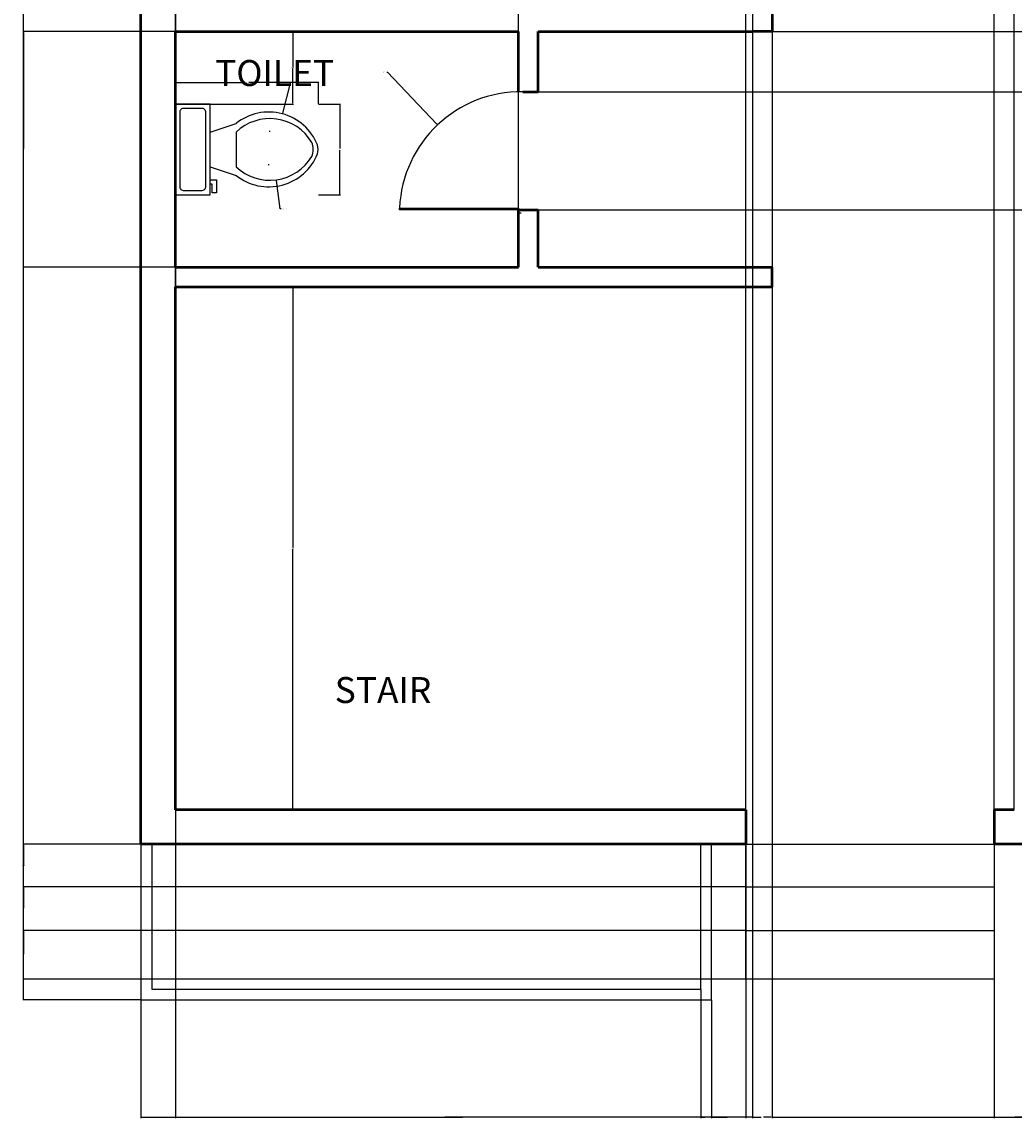
# Model space of a CAD drawing. Units: inches. Extents: x 2907 to 3328, y 1715 to 2286.
# Tile 1 of 5: x 2907 to 3137, y 1715 to 1969. Entities that reach past the tile are written whole.
import ezdxf

# ---------------------------------------------------------------- set-up
doc = ezdxf.new("R2010")
doc.units = ezdxf.units.IN
for name, color, linetype, lineweight in [('A-ANNO-DIMS', 2, 'Continuous', 18), ('A-AREA-IDEN', 7, 'Continuous', 25), ('A-DOOR', 3, 'Continuous', 25), ('A-FLOR-FIXT', 9, 'Continuous', 25), ('A-FLOR-OTLN', 7, 'Continuous', 25), ('A-FLOR-STRS', 7, 'Continuous', 25), ('A-WALL', 7, 'Continuous', 50)]:
    doc.layers.add(name, color=color, linetype=linetype, lineweight=lineweight)
doc.styles.get("Standard").update_dxf_attribs({"font": 'arial.ttf'})
doc.dimstyles.get("Standard").update_dxf_attribs({"dimtxt": 0.18, "dimasz": 0.18, "dimexe": 0.18, "dimexo": 0.0625, "dimgap": 0.09, "dimtad": 0, "dimtih": 1, "dimtoh": 1, "dimdec": 4, "dimzin": 0, "dimdsep": 46, "dimtxsty": 'Standard', "dimcen": 0.09, "dimadec": 0, "dimazin": 0, "dimtfac": 1, "dimtdec": 4, "dimtofl": 0, "dimtmove": 0, "dimatfit": 3, "dimfxl": 1, "dimtolj": 1, "dimtzin": 0, "dimarcsym": 0})

# ---------------------------------------------------------------- blocks, each defined once
blk = doc.blocks.new('Toilet - top')
for p, q in [((9.5, -6), (9.5, -2)), ((-10, -8.5), (-8, -8.5)), ((-10, -9.5), (-10, -8.5)), ((-7, -9.5), (-10, -9.5)), ((-8, -8.5), (-8, -8)), ((-7, -8), (-7, -9.5)), ((-4, -8), (-6, -14)), ((4, -8), (6, -14)), ((4, -14), (-4, -14))]:
    blk.add_line(p, q)
blk.add_lwpolyline([(10.5, -8), (10.5, 0), (-10.5, 0), (-10.5, -8)], close=True)
for points in [[(-9.5, -2), (-9.5, -6)], [(8.5, -1), (-8.5, -1)], [(-8.5, -7), (8.5, -7)]]:
    blk.add_lwpolyline(points)
for centre, radius, start, end in [((-8.62, -1.88), 0.884, 81.8699, 188.1301), ((8.62, -1.88), 0.884, 351.8699, 98.1301), ((-8.62, -6.12), 0.884, 171.8699, 278.1301), ((8.62, -6.12), 0.884, 261.8699, 8.1301), ((3.52, -21.58), 12.17, 141.4691, 247.9714), ((4.2, -21.82), 11.33, 136.3677, 238.9468), ((-3.52, -21.58), 12.17, 292.0284, 38.5307), ((-4.2, -21.82), 11.33, 301.053, 43.6321), ((0, -27.88), 4, 245.7318, 294.2682), ((0, -29), 4, 254.8605, 285.1395)]:
    blk.add_arc(centre, radius, start, end)
blk = doc.blocks.new('*D11')
at = {"layer": 'A-ANNO-DIMS', "color": 0, "lineweight": -2, "transparency": 16777216}
for p, q in [((2942.59, 1950.14), (2942.59, 1955.22)), ((2975.64, 1950.14), (2975.64, 1955.22)), ((2942.77, 1955.04), (2958.65, 1955.04)), ((2975.46, 1955.04), (2959.58, 1955.04))]:
    blk.add_line(p, q, dxfattribs=at)
at = {"layer": 'A-ANNO-DIMS', "color": 0, "transparency": 16777216}
for points in [[(2942.77, 1955.07), (2942.77, 1955.01), (2942.59, 1955.04)], [(2975.46, 1955.07), (2975.46, 1955.01), (2975.64, 1955.04)]]:
    blk.add_solid(points, dxfattribs=at)
at = {"layer": 'Defpoints', "color": 0, "transparency": 16777216}
for p in [(2942.59, 1955.04), (2942.59, 1950.08), (2975.64, 1950.08)]:
    blk.add_point(p, dxfattribs=at)
at = {"layer": 'A-ANNO-DIMS', "color": 0, "transparency": 16777216, "insert": (2959.11, 1955.04), "char_height": 0.18, "attachment_point": 5}
blk.add_mtext('\\A1;WC 33', dxfattribs=at)
blk = doc.blocks.new('*D12')
at = {"layer": 'A-ANNO-DIMS', "color": 0, "lineweight": -2, "transparency": 16777216}
for p, q in [((2975.7, 1950.08), (2980.77, 1950.08)), ((2980.59, 1949.9), (2980.59, 1939.76)), ((2980.59, 1929.26), (2980.59, 1939.4)), ((2975.7, 1929.08), (2980.77, 1929.08))]:
    blk.add_line(p, q, dxfattribs=at)
at = {"layer": 'A-ANNO-DIMS', "color": 0, "transparency": 16777216}
for points in [[(2980.56, 1949.9), (2980.62, 1949.9), (2980.59, 1950.08)], [(2980.56, 1929.26), (2980.62, 1929.26), (2980.59, 1929.08)]]:
    blk.add_solid(points, dxfattribs=at)
at = {"layer": 'Defpoints', "color": 0, "transparency": 16777216}
for p in [(2975.64, 1950.08), (2980.59, 1950.08), (2975.64, 1929.08)]:
    blk.add_point(p, dxfattribs=at)
at = {"layer": 'A-ANNO-DIMS', "color": 0, "transparency": 16777216, "insert": (2980.59, 1939.58), "char_height": 0.18, "attachment_point": 5}
blk.add_mtext('\\A1;21', dxfattribs=at)
blk = doc.blocks.new('*D14')
at = {"layer": 'A-ANNO-DIMS', "color": 0, "lineweight": -2, "transparency": 16777216}
for p, q in [((2934.53, 2258.83), (2907.26, 2258.83)), ((2907.44, 2258.65), (2907.44, 2001.01)), ((2907.44, 1743.01), (2907.44, 2000.65)), ((2934.53, 1742.83), (2907.26, 1742.83))]:
    blk.add_line(p, q, dxfattribs=at)
at = {"layer": 'A-ANNO-DIMS', "color": 0, "transparency": 16777216}
for points in [[(2907.41, 2258.65), (2907.47, 2258.65), (2907.44, 2258.83)], [(2907.41, 1743.01), (2907.47, 1743.01), (2907.44, 1742.83)]]:
    blk.add_solid(points, dxfattribs=at)
at = {"layer": 'Defpoints', "color": 0, "transparency": 16777216}
for p in [(2907.44, 2258.83), (2934.59, 2258.83), (2934.59, 1742.83)]:
    blk.add_point(p, dxfattribs=at)
at = {"layer": 'A-ANNO-DIMS', "color": 0, "transparency": 16777216, "insert": (2907.44, 2000.83), "char_height": 0.18, "attachment_point": 5}
blk.add_mtext('\\A1;516', dxfattribs=at)
blk = doc.blocks.new('*D16')
at = {"layer": 'A-ANNO-DIMS', "color": 0, "lineweight": -2, "transparency": 16777216}
for p, q in [((2942.59, 2250.77), (2942.59, 1715.5)), ((3076.09, 2250.77), (3076.09, 1715.5)), ((2942.77, 1715.68), (3008.95, 1715.68)), ((3075.91, 1715.68), (3009.73, 1715.68))]:
    blk.add_line(p, q, dxfattribs=at)
at = {"layer": 'A-ANNO-DIMS', "color": 0, "transparency": 16777216}
for points in [[(2942.77, 1715.71), (2942.77, 1715.65), (2942.59, 1715.68)], [(3075.91, 1715.71), (3075.91, 1715.65), (3076.09, 1715.68)]]:
    blk.add_solid(points, dxfattribs=at)
at = {"layer": 'Defpoints', "color": 0, "transparency": 16777216}
for p in [(2942.59, 2250.83), (3076.09, 2250.83), (3076.09, 1715.68)]:
    blk.add_point(p, dxfattribs=at)
at = {"layer": 'A-ANNO-DIMS', "color": 0, "transparency": 16777216, "insert": (3009.34, 1715.68), "char_height": 0.18, "attachment_point": 5}
blk.add_mtext('\\A1;133.5', dxfattribs=at)
blk = doc.blocks.new('*D17')
at = {"layer": 'A-ANNO-DIMS', "color": 0, "lineweight": -2, "transparency": 16777216}
for p, q in [((3080.59, 2250.77), (3080.59, 1715.5)), ((3192.09, 2250.77), (3192.09, 1715.5)), ((3080.77, 1715.68), (3135.95, 1715.68)), ((3191.91, 1715.68), (3136.73, 1715.68))]:
    blk.add_line(p, q, dxfattribs=at)
at = {"layer": 'A-ANNO-DIMS', "color": 0, "transparency": 16777216}
for points in [[(3080.77, 1715.71), (3080.77, 1715.65), (3080.59, 1715.68)], [(3191.91, 1715.71), (3191.91, 1715.65), (3192.09, 1715.68)]]:
    blk.add_solid(points, dxfattribs=at)
at = {"layer": 'Defpoints', "color": 0, "transparency": 16777216}
for p in [(3080.59, 2250.83), (3192.09, 2250.83), (3192.09, 1715.68)]:
    blk.add_point(p, dxfattribs=at)
at = {"layer": 'A-ANNO-DIMS', "color": 0, "transparency": 16777216, "insert": (3136.34, 1715.68), "char_height": 0.18, "attachment_point": 5}
blk.add_mtext('\\A1;111.5', dxfattribs=at)
blk = doc.blocks.new('*D27')
at = {"layer": 'A-ANNO-DIMS', "color": 0, "lineweight": -2, "transparency": 16777216}
for p, q in [((2942.53, 1966.83), (2907.26, 1966.83)), ((2907.44, 1966.65), (2907.44, 1939.76)), ((2907.44, 1912.51), (2907.44, 1939.4)), ((2942.53, 1912.33), (2907.26, 1912.33))]:
    blk.add_line(p, q, dxfattribs=at)
at = {"layer": 'A-ANNO-DIMS', "color": 0, "transparency": 16777216}
for points in [[(2907.41, 1966.65), (2907.47, 1966.65), (2907.44, 1966.83)], [(2907.41, 1912.51), (2907.47, 1912.51), (2907.44, 1912.33)]]:
    blk.add_solid(points, dxfattribs=at)
at = {"layer": 'Defpoints', "color": 0, "transparency": 16777216}
for p in [(2907.44, 1966.83), (2942.59, 1966.83), (2942.59, 1912.33)]:
    blk.add_point(p, dxfattribs=at)
at = {"layer": 'A-ANNO-DIMS', "color": 0, "transparency": 16777216, "insert": (2907.44, 1939.58), "char_height": 0.18, "attachment_point": 5}
blk.add_mtext('\\A1;54.5', dxfattribs=at)
blk = doc.blocks.new('*D31')
at = {"layer": 'A-ANNO-DIMS', "color": 0, "lineweight": -2, "transparency": 16777216}
for p, q in [((2942.59, 1912.39), (2942.59, 2286.16)), ((2942.77, 2285.98), (2981.88, 2285.98)), ((3021.78, 2285.98), (2982.67, 2285.98)), ((3021.96, 1912.39), (3021.96, 2286.16))]:
    blk.add_line(p, q, dxfattribs=at)
at = {"layer": 'A-ANNO-DIMS', "color": 0, "transparency": 16777216}
for points in [[(2942.77, 2286.01), (2942.77, 2285.95), (2942.59, 2285.98)], [(3021.78, 2286.01), (3021.78, 2285.95), (3021.96, 2285.98)]]:
    blk.add_solid(points, dxfattribs=at)
at = {"layer": 'Defpoints', "color": 0, "transparency": 16777216}
for p in [(3021.96, 2285.98), (2942.59, 1912.33), (3021.96, 1912.33)]:
    blk.add_point(p, dxfattribs=at)
at = {"layer": 'A-ANNO-DIMS', "color": 0, "transparency": 16777216, "insert": (2982.27, 2285.98), "char_height": 0.18, "attachment_point": 5}
blk.add_mtext('\\A1;79.37', dxfattribs=at)
blk = doc.blocks.new('*D33')
at = {"layer": 'A-ANNO-DIMS', "color": 0, "lineweight": -2, "transparency": 16777216}
for p, q in [((2934.59, 1778.77), (2934.59, 1715.5)), ((3074.5, 1778.77), (3074.5, 1715.5)), ((2934.77, 1715.68), (3004.16, 1715.68)), ((3074.32, 1715.68), (3004.93, 1715.68))]:
    blk.add_line(p, q, dxfattribs=at)
at = {"layer": 'A-ANNO-DIMS', "color": 0, "transparency": 16777216}
for points in [[(2934.77, 1715.71), (2934.77, 1715.65), (2934.59, 1715.68)], [(3074.32, 1715.71), (3074.32, 1715.65), (3074.5, 1715.68)]]:
    blk.add_solid(points, dxfattribs=at)
at = {"layer": 'Defpoints', "color": 0, "transparency": 16777216}
for p in [(2934.59, 1778.83), (3074.5, 1778.83), (3074.5, 1715.68)]:
    blk.add_point(p, dxfattribs=at)
at = {"layer": 'A-ANNO-DIMS', "color": 0, "transparency": 16777216, "insert": (3004.54, 1715.68), "char_height": 0.18, "attachment_point": 5}
blk.add_mtext('\\A1;139.9', dxfattribs=at)
blk = doc.blocks.new('*D34')
at = {"layer": 'A-ANNO-DIMS', "color": 0, "lineweight": -2, "transparency": 16777216}
for p, q in [((3074.5, 1778.89), (3074.5, 2286.16)), ((3074.68, 2285.98), (3102.84, 2285.98)), ((3131.79, 2285.98), (3103.63, 2285.98)), ((3131.97, 1778.89), (3131.97, 2286.16))]:
    blk.add_line(p, q, dxfattribs=at)
at = {"layer": 'A-ANNO-DIMS', "color": 0, "transparency": 16777216}
for points in [[(3074.68, 2286.01), (3074.68, 2285.95), (3074.5, 2285.98)], [(3131.79, 2286.01), (3131.79, 2285.95), (3131.97, 2285.98)]]:
    blk.add_solid(points, dxfattribs=at)
at = {"layer": 'Defpoints', "color": 0, "transparency": 16777216}
for p in [(3131.97, 2285.98), (3074.5, 1778.83), (3131.97, 1778.83)]:
    blk.add_point(p, dxfattribs=at)
at = {"layer": 'A-ANNO-DIMS', "color": 0, "transparency": 16777216, "insert": (3103.24, 2285.98), "char_height": 0.18, "attachment_point": 5}
blk.add_mtext('\\A1;57.47', dxfattribs=at)
blk = doc.blocks.new('*D35')
at = {"layer": 'A-ANNO-DIMS', "color": 0, "lineweight": -2, "transparency": 16777216}
for p, q in [((3131.97, 1778.77), (3131.97, 1715.5)), ((3196.08, 1778.77), (3196.08, 1715.5)), ((3132.15, 1715.68), (3163.72, 1715.68)), ((3195.9, 1715.68), (3164.33, 1715.68))]:
    blk.add_line(p, q, dxfattribs=at)
at = {"layer": 'A-ANNO-DIMS', "color": 0, "transparency": 16777216}
for points in [[(3132.15, 1715.71), (3132.15, 1715.65), (3131.97, 1715.68)], [(3195.9, 1715.71), (3195.9, 1715.65), (3196.08, 1715.68)]]:
    blk.add_solid(points, dxfattribs=at)
at = {"layer": 'Defpoints', "color": 0, "transparency": 16777216}
for p in [(3131.97, 1778.83), (3196.08, 1778.83), (3196.08, 1715.68)]:
    blk.add_point(p, dxfattribs=at)
at = {"layer": 'A-ANNO-DIMS', "color": 0, "transparency": 16777216, "insert": (3164.03, 1715.68), "char_height": 0.18, "attachment_point": 5}
blk.add_mtext('\\A1;64.1', dxfattribs=at)
blk = doc.blocks.new('*D40')
at = {"layer": 'A-ANNO-DIMS', "color": 0, "lineweight": -2, "transparency": 16777216}
for p, q in [((3026.52, 1952.9), (3327.92, 1952.9)), ((3327.74, 1952.72), (3327.74, 1939.45)), ((3327.74, 1925.82), (3327.74, 1939.09)), ((3026.52, 1925.64), (3327.92, 1925.64))]:
    blk.add_line(p, q, dxfattribs=at)
at = {"layer": 'A-ANNO-DIMS', "color": 0, "transparency": 16777216}
for points in [[(3327.71, 1952.72), (3327.77, 1952.72), (3327.74, 1952.9)], [(3327.71, 1925.82), (3327.77, 1925.82), (3327.74, 1925.64)]]:
    blk.add_solid(points, dxfattribs=at)
at = {"layer": 'Defpoints', "color": 0, "transparency": 16777216}
for p in [(3026.46, 1952.9), (3327.74, 1952.9), (3026.46, 1925.64)]:
    blk.add_point(p, dxfattribs=at)
at = {"layer": 'A-ANNO-DIMS', "color": 0, "transparency": 16777216, "insert": (3327.74, 1939.27), "char_height": 0.18, "attachment_point": 5}
blk.add_mtext('\\A1;27.27', dxfattribs=at)
blk = doc.blocks.new('*D41')
at = {"layer": 'A-ANNO-DIMS', "color": 0, "lineweight": -2, "transparency": 16777216}
for p, q in [((3026.52, 1966.83), (3327.92, 1966.83)), ((3327.74, 1966.65), (3327.74, 1960.05)), ((3327.74, 1953.08), (3327.74, 1959.68)), ((3026.52, 1952.9), (3327.92, 1952.9))]:
    blk.add_line(p, q, dxfattribs=at)
at = {"layer": 'A-ANNO-DIMS', "color": 0, "transparency": 16777216}
for points in [[(3327.71, 1966.65), (3327.77, 1966.65), (3327.74, 1966.83)], [(3327.71, 1953.08), (3327.77, 1953.08), (3327.74, 1952.9)]]:
    blk.add_solid(points, dxfattribs=at)
at = {"layer": 'Defpoints', "color": 0, "transparency": 16777216}
for p in [(3026.46, 1966.83), (3327.74, 1966.83), (3026.46, 1952.9)]:
    blk.add_point(p, dxfattribs=at)
at = {"layer": 'A-ANNO-DIMS', "color": 0, "transparency": 16777216, "insert": (3327.74, 1959.87), "char_height": 0.18, "attachment_point": 5}
blk.add_mtext('\\A1;13.927', dxfattribs=at)
blk = doc.blocks.new('*D47')
at = {"layer": 'A-ANNO-DIMS', "color": 0, "lineweight": -2, "transparency": 16777216}
for p, q in [((3076.09, 2250.77), (3076.09, 1715.5)), ((3080.59, 2250.77), (3080.59, 1715.5)), ((3076.27, 1715.68), (3078.08, 1715.68)), ((3080.41, 1715.68), (3078.6, 1715.68))]:
    blk.add_line(p, q, dxfattribs=at)
at = {"layer": 'A-ANNO-DIMS', "color": 0, "transparency": 16777216}
for points in [[(3076.27, 1715.71), (3076.27, 1715.65), (3076.09, 1715.68)], [(3080.41, 1715.71), (3080.41, 1715.65), (3080.59, 1715.68)]]:
    blk.add_solid(points, dxfattribs=at)
at = {"layer": 'Defpoints', "color": 0, "transparency": 16777216}
for p in [(3076.09, 2250.83), (3080.59, 2250.83), (3080.59, 1715.68)]:
    blk.add_point(p, dxfattribs=at)
at = {"layer": 'A-ANNO-DIMS', "color": 0, "transparency": 16777216, "insert": (3078.34, 1715.68), "char_height": 0.18, "attachment_point": 5}
blk.add_mtext('\\A1;4.5', dxfattribs=at)
blk = doc.blocks.new('*D48')
at = {"layer": 'A-ANNO-DIMS', "color": 0, "lineweight": -2, "transparency": 16777216}
for p, q in [((3074.5, 1747.6), (3074.5, 1715.5)), ((3066.59, 1742.77), (3066.59, 1715.5)), ((3066.77, 1715.68), (3070.24, 1715.68)), ((3074.32, 1715.68), (3070.85, 1715.68))]:
    blk.add_line(p, q, dxfattribs=at)
at = {"layer": 'A-ANNO-DIMS', "color": 0, "transparency": 16777216}
for points in [[(3066.77, 1715.71), (3066.77, 1715.65), (3066.59, 1715.68)], [(3074.32, 1715.71), (3074.32, 1715.65), (3074.5, 1715.68)]]:
    blk.add_solid(points, dxfattribs=at)
at = {"layer": 'Defpoints', "color": 0, "transparency": 16777216}
for p in [(3074.5, 1747.67), (3066.59, 1742.83), (3074.5, 1715.68)]:
    blk.add_point(p, dxfattribs=at)
at = {"layer": 'A-ANNO-DIMS', "color": 0, "transparency": 16777216, "insert": (3070.54, 1715.68), "char_height": 0.18, "attachment_point": 5}
blk.add_mtext('\\A1;7.91', dxfattribs=at)
blk = doc.blocks.new('*D49')
at = {"layer": 'A-ANNO-DIMS', "color": 0, "lineweight": -2, "transparency": 16777216}
for p, q in [((3131.97, 1747.6), (3131.97, 1715.5)), ((3144.59, 1742.77), (3144.59, 1715.5)), ((3132.15, 1715.68), (3137.83, 1715.68)), ((3144.41, 1715.68), (3138.74, 1715.68))]:
    blk.add_line(p, q, dxfattribs=at)
at = {"layer": 'A-ANNO-DIMS', "color": 0, "transparency": 16777216}
for points in [[(3132.15, 1715.71), (3132.15, 1715.65), (3131.97, 1715.68)], [(3144.41, 1715.71), (3144.41, 1715.65), (3144.59, 1715.68)]]:
    blk.add_solid(points, dxfattribs=at)
at = {"layer": 'Defpoints', "color": 0, "transparency": 16777216}
for p in [(3131.97, 1747.67), (3144.59, 1742.83), (3144.59, 1715.68)]:
    blk.add_point(p, dxfattribs=at)
at = {"layer": 'A-ANNO-DIMS', "color": 0, "transparency": 16777216, "insert": (3138.28, 1715.68), "char_height": 0.18, "attachment_point": 5}
blk.add_mtext('\\A1;12.616', dxfattribs=at)
blk = doc.blocks.new('*D50')
at = {"layer": 'A-ANNO-DIMS', "color": 0, "lineweight": -2, "transparency": 16777216}
for p, q in [((3074.44, 1758.9), (2907.26, 1758.9)), ((2907.44, 1758.72), (2907.44, 1753.47)), ((2907.44, 1747.85), (2907.44, 1753.1)), ((3074.44, 1747.67), (2907.26, 1747.67))]:
    blk.add_line(p, q, dxfattribs=at)
at = {"layer": 'A-ANNO-DIMS', "color": 0, "transparency": 16777216}
for points in [[(2907.41, 1758.72), (2907.47, 1758.72), (2907.44, 1758.9)], [(2907.41, 1747.85), (2907.47, 1747.85), (2907.44, 1747.67)]]:
    blk.add_solid(points, dxfattribs=at)
at = {"layer": 'Defpoints', "color": 0, "transparency": 16777216}
for p in [(2907.44, 1758.9), (3074.5, 1758.9), (3074.5, 1747.67)]:
    blk.add_point(p, dxfattribs=at)
at = {"layer": 'A-ANNO-DIMS', "color": 0, "transparency": 16777216, "insert": (2907.44, 1753.29), "char_height": 0.18, "attachment_point": 5}
blk.add_mtext('\\A1;11.236', dxfattribs=at)
blk = doc.blocks.new('*D51')
at = {"layer": 'A-ANNO-DIMS', "color": 0, "lineweight": -2, "transparency": 16777216}
for p, q in [((3074.44, 1769.03), (2907.26, 1769.03)), ((2907.44, 1768.85), (2907.44, 1764.15)), ((2907.44, 1759.08), (2907.44, 1763.78)), ((3074.44, 1758.9), (2907.26, 1758.9))]:
    blk.add_line(p, q, dxfattribs=at)
at = {"layer": 'A-ANNO-DIMS', "color": 0, "transparency": 16777216}
for points in [[(2907.41, 1768.85), (2907.47, 1768.85), (2907.44, 1769.03)], [(2907.41, 1759.08), (2907.47, 1759.08), (2907.44, 1758.9)]]:
    blk.add_solid(points, dxfattribs=at)
at = {"layer": 'Defpoints', "color": 0, "transparency": 16777216}
for p in [(2907.44, 1769.03), (3074.5, 1769.03), (3074.5, 1758.9)]:
    blk.add_point(p, dxfattribs=at)
at = {"layer": 'A-ANNO-DIMS', "color": 0, "transparency": 16777216, "insert": (2907.44, 1763.97), "char_height": 0.18, "attachment_point": 5}
blk.add_mtext('\\A1;10.124', dxfattribs=at)
blk = doc.blocks.new('*D52')
at = {"layer": 'A-ANNO-DIMS', "color": 0, "lineweight": -2, "transparency": 16777216}
for p, q in [((3074.44, 1778.83), (2907.26, 1778.83)), ((2907.44, 1778.65), (2907.44, 1774.11)), ((2907.44, 1769.21), (2907.44, 1773.75)), ((3074.44, 1769.03), (2907.26, 1769.03))]:
    blk.add_line(p, q, dxfattribs=at)
at = {"layer": 'A-ANNO-DIMS', "color": 0, "transparency": 16777216}
for points in [[(2907.41, 1778.65), (2907.47, 1778.65), (2907.44, 1778.83)], [(2907.41, 1769.21), (2907.47, 1769.21), (2907.44, 1769.03)]]:
    blk.add_solid(points, dxfattribs=at)
at = {"layer": 'Defpoints', "color": 0, "transparency": 16777216}
for p in [(2907.44, 1778.83), (3074.5, 1778.83), (3074.5, 1769.03)]:
    blk.add_point(p, dxfattribs=at)
at = {"layer": 'A-ANNO-DIMS', "color": 0, "transparency": 16777216, "insert": (2907.44, 1773.93), "char_height": 0.18, "attachment_point": 5}
blk.add_mtext('\\A1;9.803', dxfattribs=at)
blk = doc.blocks.new('*D53')
at = {"layer": 'A-ANNO-DIMS', "color": 0, "lineweight": -2, "transparency": 16777216}
for p, q in [((3064.09, 1745.27), (3064.09, 1715.5)), ((3066.59, 1742.77), (3066.59, 1715.5)), ((3064.27, 1715.68), (3065.08, 1715.68)), ((3066.41, 1715.68), (3065.6, 1715.68))]:
    blk.add_line(p, q, dxfattribs=at)
at = {"layer": 'A-ANNO-DIMS', "color": 0, "transparency": 16777216}
for points in [[(3064.27, 1715.71), (3064.27, 1715.65), (3064.09, 1715.68)], [(3066.41, 1715.71), (3066.41, 1715.65), (3066.59, 1715.68)]]:
    blk.add_solid(points, dxfattribs=at)
at = {"layer": 'Defpoints', "color": 0, "transparency": 16777216}
for p in [(3064.09, 1745.33), (3066.59, 1742.83), (3066.59, 1715.68)]:
    blk.add_point(p, dxfattribs=at)
at = {"layer": 'A-ANNO-DIMS', "color": 0, "transparency": 16777216, "insert": (3065.34, 1715.68), "char_height": 0.18, "attachment_point": 5}
blk.add_mtext('\\A1;2.5', dxfattribs=at)
blk = doc.blocks.new('*D54')
at = {"layer": 'A-ANNO-DIMS', "color": 0, "lineweight": -2, "transparency": 16777216}
for p, q in [((2942.65, 1907.83), (2969.92, 1907.83)), ((2969.74, 1907.65), (2969.74, 1847.51)), ((2969.74, 1787.01), (2969.74, 1847.15)), ((2942.65, 1786.83), (2969.92, 1786.83))]:
    blk.add_line(p, q, dxfattribs=at)
at = {"layer": 'A-ANNO-DIMS', "color": 0, "transparency": 16777216}
for points in [[(2969.71, 1907.65), (2969.77, 1907.65), (2969.74, 1907.83)], [(2969.71, 1787.01), (2969.77, 1787.01), (2969.74, 1786.83)]]:
    blk.add_solid(points, dxfattribs=at)
at = {"layer": 'Defpoints', "color": 0, "transparency": 16777216}
for p in [(2942.59, 1907.83), (2942.59, 1786.83), (2969.74, 1786.83)]:
    blk.add_point(p, dxfattribs=at)
at = {"layer": 'A-ANNO-DIMS', "color": 0, "transparency": 16777216, "insert": (2969.74, 1847.33), "char_height": 0.18, "attachment_point": 5}
blk.add_mtext('\\A1;121', dxfattribs=at)
blk = doc.blocks.new('*D55')
at = {"layer": 'A-ANNO-DIMS', "color": 0, "lineweight": -2, "transparency": 16777216}
for p, q in [((2942.65, 1966.83), (2969.92, 1966.83)), ((2969.74, 1966.65), (2969.74, 1958.64)), ((2969.74, 1950.26), (2969.74, 1958.27)), ((2942.65, 1950.08), (2969.92, 1950.08))]:
    blk.add_line(p, q, dxfattribs=at)
at = {"layer": 'A-ANNO-DIMS', "color": 0, "transparency": 16777216}
for points in [[(2969.71, 1966.65), (2969.77, 1966.65), (2969.74, 1966.83)], [(2969.71, 1950.26), (2969.77, 1950.26), (2969.74, 1950.08)]]:
    blk.add_solid(points, dxfattribs=at)
at = {"layer": 'Defpoints', "color": 0, "transparency": 16777216}
for p in [(2942.59, 1966.83), (2942.59, 1950.08), (2969.74, 1950.08)]:
    blk.add_point(p, dxfattribs=at)
at = {"layer": 'A-ANNO-DIMS', "color": 0, "transparency": 16777216, "insert": (2969.74, 1958.46), "char_height": 0.18, "attachment_point": 5}
blk.add_mtext('\\A1;16.75', dxfattribs=at)
blk = doc.blocks.new('*D56')
at = {"layer": 'A-ANNO-DIMS', "color": 0, "lineweight": -2, "transparency": 16777216}
for p, q in [((2942.59, 1786.89), (2942.59, 2286.16)), ((2942.77, 2285.98), (3039.31, 2285.98)), ((3136.41, 2285.98), (3039.87, 2285.98)), ((3136.59, 1786.89), (3136.59, 2286.16))]:
    blk.add_line(p, q, dxfattribs=at)
at = {"layer": 'A-ANNO-DIMS', "color": 0, "transparency": 16777216}
for points in [[(2942.77, 2286.01), (2942.77, 2285.95), (2942.59, 2285.98)], [(3136.41, 2286.01), (3136.41, 2285.95), (3136.59, 2285.98)]]:
    blk.add_solid(points, dxfattribs=at)
at = {"layer": 'Defpoints', "color": 0, "transparency": 16777216}
for p in [(3136.59, 2285.98), (2942.59, 1786.83), (3136.59, 1786.83)]:
    blk.add_point(p, dxfattribs=at)
at = {"layer": 'A-ANNO-DIMS', "color": 0, "transparency": 16777216, "insert": (3039.59, 2285.98), "char_height": 0.18, "attachment_point": 5}
blk.add_mtext('\\A1;194', dxfattribs=at)
blk = doc.blocks.new('*D60')
at = {"layer": 'A-ANNO-DIMS', "color": 0, "lineweight": -2, "transparency": 16777216}
for p, q in [((2991.47, 1957.49), (2991.65, 1957.49)), ((2991.65, 1957.49), (3003.07, 1945.39)), ((3022.35, 1924.88), (3022.53, 1924.88)), ((3022.44, 1924.79), (3022.44, 1924.97))]:
    blk.add_line(p, q, dxfattribs=at)
at = {"layer": 'A-ANNO-DIMS', "color": 0, "transparency": 16777216}
blk.add_solid([(3003.09, 1945.41), (3003.05, 1945.37), (3003.19, 1945.26)], dxfattribs=at)
at = {"layer": 'Defpoints', "color": 0, "transparency": 16777216}
for p in [(3003.19, 1945.26), (3022.44, 1924.88)]:
    blk.add_point(p, dxfattribs=at)
at = {"layer": 'A-ANNO-DIMS', "color": 0, "transparency": 16777216, "insert": (2990.99, 1957.49), "char_height": 0.18, "attachment_point": 5}
blk.add_mtext('\\A1;R28.03', dxfattribs=at)
blk = doc.blocks.new('*D63')
at = {"layer": 'A-ANNO-DIMS', "color": 0, "lineweight": -2, "transparency": 16777216}
for p, q in [((2969.12, 1954.89), (2967.31, 1948)), ((2969.3, 1954.89), (2969.12, 1954.89)), ((2964.08, 1936.06), (2964.26, 1936.06)), ((2964.17, 1935.97), (2964.17, 1936.15))]:
    blk.add_line(p, q, dxfattribs=at)
at = {"layer": 'A-ANNO-DIMS', "color": 0, "transparency": 16777216}
blk.add_solid([(2967.28, 1948.01), (2967.34, 1948), (2967.26, 1947.83)], dxfattribs=at)
at = {"layer": 'Defpoints', "color": 0, "transparency": 16777216}
for p in [(2967.26, 1947.83), (2964.17, 1936.06)]:
    blk.add_point(p, dxfattribs=at)
at = {"layer": 'A-ANNO-DIMS', "color": 0, "transparency": 16777216, "insert": (2969.97, 1954.89), "char_height": 0.18, "attachment_point": 5}
blk.add_mtext('\\A1;2X R12.17', dxfattribs=at)
blk = doc.blocks.new('*D64')
at = {"layer": 'A-ANNO-DIMS', "color": 0, "lineweight": -2, "transparency": 16777216}
for p, q in [((2964.32, 1943.78), (2964.5, 1943.78)), ((2964.41, 1943.69), (2964.41, 1943.87)), ((2966.82, 1925.81), (2965.94, 1932.37)), ((2967, 1925.81), (2966.82, 1925.81))]:
    blk.add_line(p, q, dxfattribs=at)
at = {"layer": 'A-ANNO-DIMS', "color": 0, "transparency": 16777216}
blk.add_solid([(2965.97, 1932.38), (2965.91, 1932.37), (2965.92, 1932.55)], dxfattribs=at)
at = {"layer": 'Defpoints', "color": 0, "transparency": 16777216}
for p in [(2964.41, 1943.78), (2965.92, 1932.55)]:
    blk.add_point(p, dxfattribs=at)
at = {"layer": 'A-ANNO-DIMS', "color": 0, "transparency": 16777216, "insert": (2967.68, 1925.81), "char_height": 0.18, "attachment_point": 5}
blk.add_mtext('\\A1;2X R11.33', dxfattribs=at)

msp = doc.modelspace()

# ---------------------------------------------------------------- linework, layer by layer
at = {"layer": 'A-DOOR'}
for p, q in [((2994.4311, 1925.6352), (2994.4311, 1926.0068)), ((2994.4311, 1926.0068), (3021.96, 1926.0068)), ((3021.96, 1925.6352), (2994.4311, 1925.6352)), ((2994.4311, 1925.6352), (2994.4311, 1925.6352)), ((3021.96, 1926.0068), (3021.96, 1925.6352))]:
    msp.add_line(p, q, dxfattribs=at)
msp.add_arc((3022.4376, 1924.8784), 28.0292, 89.023742, 177.6928, dxfattribs=at)
at = {"layer": 'A-FLOR-OTLN'}
for p, q in [((2934.5892, 1778.8301), (2934.5892, 1742.8301)), ((2937.0892, 1778.8301), (2937.0892, 1745.3301)), ((3064.0892, 1745.3301), (3064.0892, 1778.8301)), ((3066.5892, 1742.8301), (3066.5892, 1778.8301)), ((2937.0892, 1745.3301), (3064.0892, 1745.3301)), ((2934.5892, 1742.8301), (3066.5892, 1742.8301))]:
    msp.add_line(p, q, dxfattribs=at)
at = {"layer": 'A-FLOR-STRS'}
for p, q in [((3074.499, 1778.8301), (3131.9734, 1778.8301)), ((3074.499, 1747.6674), (3074.499, 1778.8301)), ((3131.9734, 1778.8301), (3131.9734, 1747.6674)), ((3074.499, 1769.0274), (3131.9734, 1769.0274)), ((3074.499, 1758.9033), (3131.9734, 1758.9033)), ((3131.9734, 1747.6674), (3074.499, 1747.6674))]:
    msp.add_line(p, q, dxfattribs=at)
at = {"layer": 'A-WALL'}
for p, q in [((2934.5892, 1778.8301), (2934.5892, 2258.8301)), ((3080.5892, 2038.1078), (3080.5892, 1966.8301)), ((2942.5892, 1966.8301), (3021.96, 1966.8301)), ((2942.5892, 1912.3301), (2942.5892, 1966.8301)), ((3021.96, 1952.9036), (3021.96, 1966.8301)), ((3026.46, 1952.9036), (3026.46, 1966.8301)), ((3026.46, 1966.8301), (3076.0892, 1966.8301)), ((3080.5892, 1966.8301), (3076.0892, 1966.8301)), ((3022.9152, 1952.9036), (3026.46, 1952.9036)), ((3021.96, 1912.3301), (3021.96, 1925.6352)), ((3021.96, 1925.6352), (3026.46, 1925.6352)), ((3026.46, 1912.3301), (3026.46, 1925.6352)), ((2942.5892, 1912.3301), (3021.96, 1912.3301)), ((3026.46, 1912.3301), (3080.5892, 1912.3301)), ((3080.5892, 1907.8301), (3080.5892, 1912.3301)), ((2942.5892, 1786.8301), (2942.5892, 1907.8301)), ((2942.5892, 1907.8301), (3080.5892, 1907.8301)), ((3074.499, 1786.8301), (2942.5892, 1786.8301)), ((3074.499, 1786.8301), (3074.499, 1778.8301)), ((3136.5892, 1786.8301), (3131.9734, 1786.8301)), ((3131.9734, 1786.8301), (3131.9734, 1778.8301)), ((3074.499, 1778.8301), (2934.5892, 1778.8301)), ((3300.5892, 1778.8301), (3131.9734, 1778.8301))]:
    msp.add_line(p, q, dxfattribs=at)

# ---------------------------------------------------------------- block references
at = {"layer": 'A-FLOR-FIXT', "rotation": 90}
msp.add_blockref('Toilet - top', (2942.5892, 1939.5801), dxfattribs=at)

# ---------------------------------------------------------------- texts
at = {"layer": 'A-AREA-IDEN', "char_height": 6, "attachment_point": 1}
for s, insert in [('TOILET ', (2951.7536, 1960.258)), ('STAIR', (2979.4206, 1817.5152))]:
    msp.add_mtext_dynamic_manual_height_columns(s, width=50.965346, gutter_width=12.5, heights=[0], dxfattribs=dict(at, insert=insert))

# ---------------------------------------------------------------- dimensions: what is measured, and where the dimension line sits
at = {"layer": 'A-ANNO-DIMS'}
for base, p1, p2, override, picture, middle in [((3021.96, 2285.9816), (2942.5892, 1912.3301), (3021.96, 1912.3301), {"dimdec": 2, "dimlfac": 1, "dimrnd": 0, "dimzin": 0, "dimdsep": 46, "dimlunit": 2}, '*D31', (2982.2746, 2285.9816)), ((3136.5892, 2285.9816), (2942.5892, 1786.8301), (3136.5892, 1786.8301), {"dimdec": 0, "dimlfac": 1, "dimrnd": 0, "dimzin": 0, "dimdsep": 46, "dimlunit": 2}, '*D56', (3039.5892, 2285.9816)), ((3131.9734, 2285.9816), (3074.499, 1778.8301), (3131.9734, 1778.8301), {"dimdec": 2, "dimlfac": 1, "dimrnd": 0, "dimzin": 0, "dimdsep": 46, "dimlunit": 2}, '*D34', (3103.2362, 2285.9816)), ((3076.0892, 1715.6786), (2942.5892, 2250.8301), (3076.0892, 2250.8301), {"dimdec": 1, "dimlfac": 1, "dimrnd": 0, "dimzin": 0, "dimdsep": 46, "dimlunit": 2}, '*D16', (3009.3392, 1715.6786)), ((3080.5892, 1715.6786), (3076.0892, 2250.8301), (3080.5892, 2250.8301), {"dimdec": 1, "dimlfac": 1, "dimrnd": 0, "dimzin": 0, "dimdsep": 46, "dimlunit": 2}, '*D47', (3078.3392, 1715.6786)), ((3192.0892, 1715.6786), (3080.5892, 2250.8301), (3192.0892, 2250.8301), {"dimdec": 1, "dimlfac": 1, "dimrnd": 0, "dimzin": 0, "dimdsep": 46, "dimlunit": 2}, '*D17', (3136.3392, 1715.6786)), ((3074.499, 1715.6786), (2934.5892, 1778.8301), (3074.499, 1778.8301), {"dimdec": 1, "dimlfac": 1, "dimrnd": 0, "dimzin": 0, "dimdsep": 46, "dimlunit": 2}, '*D33', (3004.5441, 1715.6786)), ((3196.0778, 1715.6786), (3131.9734, 1778.8301), (3196.0778, 1778.8301), {"dimdec": 1, "dimlfac": 1, "dimrnd": 0, "dimzin": 0, "dimdsep": 46, "dimlunit": 2}, '*D35', (3164.0256, 1715.6786)), ((3074.499, 1715.6786), (3066.5892, 1742.8301), (3074.499, 1747.6674), {"dimdec": 2, "dimlfac": 1, "dimrnd": 0, "dimzin": 0, "dimdsep": 46, "dimlunit": 2}, '*D48', (3070.5441, 1715.6786)), ((3144.5892, 1715.6786), (3131.9734, 1747.6674), (3144.5892, 1742.8301), {"dimdec": 3, "dimlfac": 1, "dimrnd": 0, "dimzin": 0, "dimdsep": 46, "dimlunit": 2}, '*D49', (3138.2813, 1715.6786)), ((3066.5892, 1715.6786), (3064.0892, 1745.3301), (3066.5892, 1742.8301), {"dimdec": 1, "dimlfac": 1, "dimrnd": 0, "dimzin": 0, "dimdsep": 46, "dimlunit": 2}, '*D53', (3065.3392, 1715.6786))]:
    dim = msp.add_linear_dim(base=base, p1=p1, p2=p2, dimstyle='Standard', override=override, dxfattribs=at)
    dim.commit()
    dim.dimension.update_dxf_attribs({"geometry": picture, "text_midpoint": middle})
for base, p1, p2, angle, override, picture, middle in [((2907.4377, 2258.8301), (2934.5892, 1742.8301), (2934.5892, 2258.8301), 90, {"dimdec": 0, "dimlfac": 1, "dimrnd": 0, "dimzin": 0, "dimdsep": 46, "dimlunit": 2}, '*D14', (2907.4377, 2000.8301)), ((2907.4377, 1966.8301), (2942.5892, 1912.3301), (2942.5892, 1966.8301), 90, {"dimdec": 1, "dimlfac": 1, "dimrnd": 0, "dimzin": 0, "dimdsep": 46, "dimlunit": 2}, '*D27', (2907.4377, 1939.5801)), ((2969.7407, 1950.0801), (2942.5892, 1966.8301), (2942.5892, 1950.0801), 270, {"dimdec": 2, "dimlfac": 1, "dimrnd": 0, "dimzin": 0, "dimdsep": 46, "dimlunit": 2}, '*D55', (2969.7407, 1958.4551)), ((3327.74068, 1966.8301), (3026.46005, 1952.90358), (3026.46005, 1966.8301), 90, {"dimdec": 3, "dimlfac": 1, "dimrnd": 0, "dimzin": 0, "dimdsep": 46, "dimlunit": 2}, '*D41', (3327.74068, 1959.86684)), ((3327.7407, 1952.9036), (3026.46, 1925.6352), (3026.46, 1952.9036), 90, {"dimdec": 2, "dimlfac": 1, "dimrnd": 0, "dimzin": 0, "dimdsep": 46, "dimlunit": 2}, '*D40', (3327.7407, 1939.2694)), ((2980.5924, 1950.0801), (2975.6354, 1929.0801), (2975.6354, 1950.0801), 90, {"dimdec": 0, "dimlfac": 1, "dimrnd": 0, "dimzin": 0, "dimdsep": 46, "dimlunit": 2}, '*D12', (2980.5924, 1939.5801)), ((2969.7407, 1786.8301), (2942.5892, 1907.8301), (2942.5892, 1786.8301), 270, {"dimdec": 0, "dimlfac": 1, "dimrnd": 0, "dimzin": 0, "dimdsep": 46, "dimlunit": 2}, '*D54', (2969.7407, 1847.3301)), ((2907.4377, 1778.8301), (3074.499, 1769.0274), (3074.499, 1778.8301), 90, {"dimdec": 3, "dimlfac": 1, "dimrnd": 0, "dimzin": 0, "dimdsep": 46, "dimlunit": 2}, '*D52', (2907.4377, 1773.9287)), ((2907.4377, 1769.0274), (3074.499, 1758.9033), (3074.499, 1769.0274), 90, {"dimdec": 3, "dimlfac": 1, "dimrnd": 0, "dimzin": 0, "dimdsep": 46, "dimlunit": 2}, '*D51', (2907.4377, 1763.9654)), ((2907.4377, 1758.9033), (3074.499, 1747.6674), (3074.499, 1758.9033), 90, {"dimdec": 3, "dimlfac": 1, "dimrnd": 0, "dimzin": 0, "dimdsep": 46, "dimlunit": 2}, '*D50', (2907.4377, 1753.2854))]:
    dim = msp.add_linear_dim(base=base, p1=p1, p2=p2, angle=angle, dimstyle='Standard', override=override, dxfattribs=at)
    dim.commit()
    dim.dimension.update_dxf_attribs({"geometry": picture, "text_midpoint": middle})
dim = msp.add_linear_dim(base=(2942.5892, 1955.037), p1=(2975.6354, 1950.0801), p2=(2942.5892, 1950.0801), angle=180, text='WC <>', dimstyle='Standard', override={"dimdec": 0, "dimlfac": 1, "dimrnd": 0, "dimzin": 0, "dimdsep": 46, "dimlunit": 2}, dxfattribs=at)
dim.commit()
dim.dimension.update_dxf_attribs({"geometry": '*D11', "text_midpoint": (2959.1123, 1955.037)})
for center, mpoint, picture, middle in [((2964.1697, 1936.0606), (2967.262, 1947.8302), '*D63', (2969.9722, 1954.8919)), ((2964.4066, 1943.7801), (2965.916, 1932.5519), '*D64', (2967.6764, 1925.815))]:
    dim = msp.add_radius_dim(center=center, mpoint=mpoint, text='2X <>', dimstyle='Standard', override={"dimdec": 2, "dimlfac": 1, "dimrnd": 0, "dimzin": 0, "dimdsep": 46, "dimlunit": 2}, dxfattribs=at)
    dim.commit()
    dim.dimension.update_dxf_attribs({"geometry": picture, "text_midpoint": middle, "dimtype": 164})
dim = msp.add_radius_dim(center=(3022.4376, 1924.8784), mpoint=(3003.1941, 1945.2579), dimstyle='Standard', override={"dimdec": 2, "dimlfac": 1, "dimrnd": 0, "dimzin": 0, "dimdsep": 46, "dimlunit": 2}, dxfattribs=at)
dim.commit()
dim.dimension.update_dxf_attribs({"geometry": '*D60', "text_midpoint": (2990.9881, 1957.4856), "dimtype": 164})

doc.saveas('drawing.dxf')
